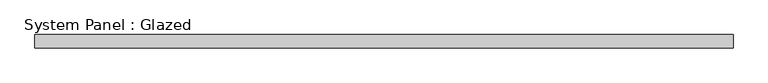
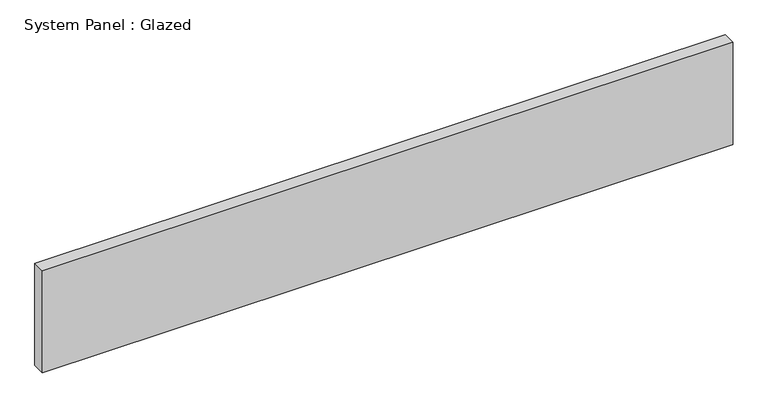
"""IFC4 building model written with IfcOpenShell, lengths in millimetres: plate geometry, System Panel : Glazed."""

from ifc_helpers import new_model, si_unit, origin, origin_with_axes, place, context, project, spatial, polyline, outline, extrude, source, transform, mapped, element, save


def system_panel_glazed_f3e19b1d(model_context):
    return source(origin(), model_context, "Body", "SweptSolid", [
        extrude(outline(polyline([(669.925, 19.05), (-669.925, 19.05), (-669.925, 44.45), (669.925, 44.45), (669.925, 19.05)])), origin_with_axes(), (0.0, 0.0, 1.0), 209.55),
    ])


if __name__ == "__main__":
    model = new_model("IFC4")
    model_context = context("Model", 3, world=origin())
    ifc_project = project(units=[si_unit("LENGTHUNIT", "METRE", prefix="MILLI")], contexts=[model_context])
    site = spatial("IfcSite", under=ifc_project)
    building = spatial("IfcBuilding", under=site)
    placement = place(None, origin())
    system_panel_glazed_shape = system_panel_glazed_f3e19b1d(model_context)
    element("IfcPlate", 1, ObjectType="System Panel : Glazed", at=placement, inside=building, context=model_context, shape_type="MappedRepresentation", body=[
        mapped(system_panel_glazed_shape, transform((0.0, 0.0, 0.0), x_axis=(1.0, 0.0, 0.0), y_axis=(0.0, 1.0, 0.0), z_axis=(0.0, 0.0, 1.0))),
    ])
    save(model, "model.ifc")

# Revit data of these elements
# Type "System Panel : Glazed"
#   Construction Type Id = "GSP4R"
#   Analytic Construction = "1/8 in Pilkington single glazing"
#   Visual Light Transmittance = 0.9
#   Solar Heat Gain Coefficient = 0.86
#   Heat Transfer Coefficient (U) = 1.18115 BTU/(h·ft²·°F)
#   Define Thermal Properties by = 1
# Element 1 (IfcPlate, "System Panel : Glazed")
#   Materials on its faces: "Glass"
# Materials
#   "Glass": class "Glass", colour RGB 0 128 192, transparency 0.75, Description = "Soda Lime Glass", Cost = 0
